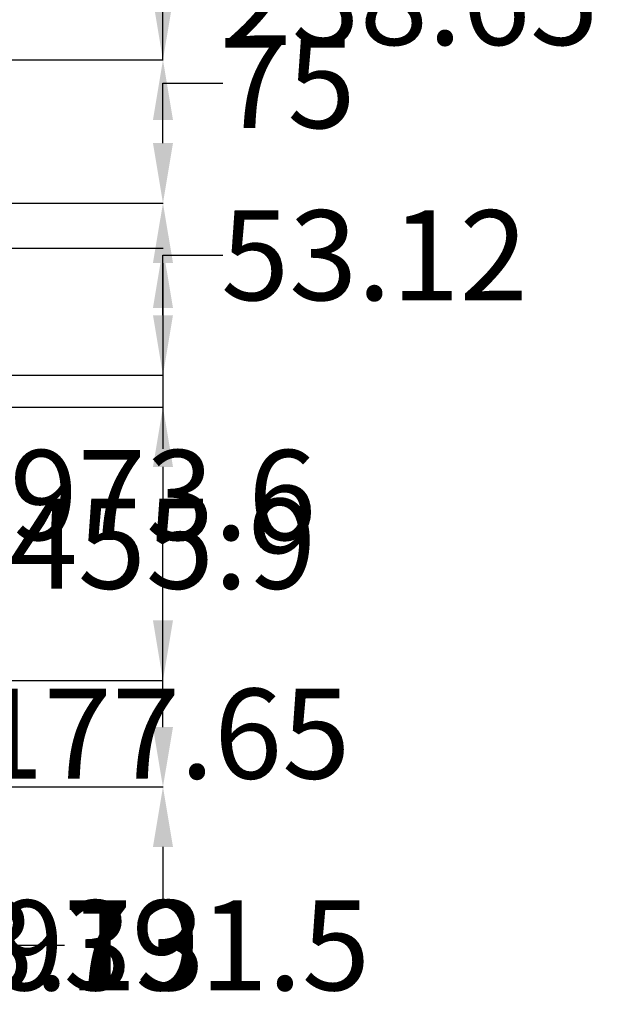
# Model space of a CAD drawing. Units: millimetres. Extents: x -504 to 6314, y 1290 to 4335.
# Tile 8 of 9: x 5350 to 6314, y 1290 to 2932. Entities that reach past the tile are written whole.
import ezdxf

# ---------------------------------------------------------------- set-up
doc = ezdxf.new("R2010")
doc.units = ezdxf.units.MM
doc.header["$MEASUREMENT"] = 0
doc.layers.add('A-ANNO-DIMS', color=2, linetype='Continuous', lineweight=18)
doc.styles.get("Standard").update_dxf_attribs({"font": 'arial.ttf'})
doc.dimstyles.get("Standard").update_dxf_attribs({"dimtxt": 150, "dimasz": 100, "dimexe": 0.18, "dimexo": 0.0625, "dimgap": 0.09, "dimtad": 0, "dimtih": 1, "dimtoh": 1, "dimdec": 0, "dimzin": 0, "dimdsep": 46, "dimtxsty": 'Standard', "dimcen": 0.09, "dimadec": 0, "dimazin": 0, "dimtfac": 1, "dimtdec": 0, "dimtofl": 0, "dimtmove": 0, "dimatfit": 3, "dimfxl": 1, "dimtolj": 1, "dimtzin": 0, "dimarcsym": 0})

# ---------------------------------------------------------------- blocks, each defined once
blk = doc.blocks.new('*D5')
at = {"layer": 'A-ANNO-DIMS', "color": 0, "lineweight": -2, "transparency": 16777216}
for p, q in [((4260.1, 2625.8), (5589, 2625.8)), ((5588.8, 2525.8), (5588.8, 2215.7)), ((5588.8, 1752.1), (5588.8, 2062.2)), ((72.9, 1652.1), (5589, 1652.1))]:
    blk.add_line(p, q, dxfattribs=at)
at = {"layer": 'A-ANNO-DIMS', "color": 0, "transparency": 16777216}
for points in [[(5572.1, 2525.8), (5605.5, 2525.8), (5588.8, 2625.8)], [(5572.1, 1752.1), (5605.5, 1752.1), (5588.8, 1652.1)]]:
    blk.add_solid(points, dxfattribs=at)
at = {"layer": 'Defpoints', "color": 0, "transparency": 16777216}
for p in [(4260, 2625.8), (5588.8, 2625.8), (72.8, 1652.1)]:
    blk.add_point(p, dxfattribs=at)
at = {"layer": 'A-ANNO-DIMS', "color": 0, "transparency": 16777216, "insert": (5588.8, 2138.9), "char_height": 150, "attachment_point": 5}
blk.add_mtext('\\A1;973.6', dxfattribs=at)
blk = doc.blocks.new('*D27')
at = {"layer": 'A-ANNO-DIMS', "color": 0, "lineweight": -2, "transparency": 16777216}
for p, q in [((5588.8, 3138.9), (5588.8, 3238.9)), ((5588.8, 3238.9), (5688.8, 3238.9)), ((5081.2, 3138.9), (5589, 3138.9)), ((5588.8, 2964.4), (5588.8, 3038.9)), ((4489, 2864.4), (5589, 2864.4))]:
    blk.add_line(p, q, dxfattribs=at)
at = {"layer": 'A-ANNO-DIMS', "color": 0, "transparency": 16777216}
for points in [[(5572.1, 3038.9), (5605.5, 3038.9), (5588.8, 3138.9)], [(5572.1, 2964.4), (5605.5, 2964.4), (5588.8, 2864.4)]]:
    blk.add_solid(points, dxfattribs=at)
at = {"layer": 'Defpoints', "color": 0, "transparency": 16777216}
for p in [(5081.2, 3138.9), (5588.8, 3138.9), (4489, 2864.4)]:
    blk.add_point(p, dxfattribs=at)
at = {"layer": 'A-ANNO-DIMS', "color": 0, "transparency": 16777216, "insert": (6001.2, 3238.9), "char_height": 150, "attachment_point": 5}
blk.add_mtext('\\A1;274.54', dxfattribs=at)
blk = doc.blocks.new('*D29')
at = {"layer": 'A-ANNO-DIMS', "color": 0, "lineweight": -2, "transparency": 16777216}
for p, q in [((5588.8, 2864.4), (5588.8, 2964.4)), ((5588.8, 2964.4), (5688.8, 2964.4)), ((4489, 2864.4), (5589, 2864.4)), ((5588.8, 2725.8), (5588.8, 2764.4)), ((4260.1, 2625.8), (5589, 2625.8))]:
    blk.add_line(p, q, dxfattribs=at)
at = {"layer": 'A-ANNO-DIMS', "color": 0, "transparency": 16777216}
for points in [[(5572.1, 2764.4), (5605.5, 2764.4), (5588.8, 2864.4)], [(5572.1, 2725.8), (5605.5, 2725.8), (5588.8, 2625.8)]]:
    blk.add_solid(points, dxfattribs=at)
at = {"layer": 'Defpoints', "color": 0, "transparency": 16777216}
for p in [(4489, 2864.4), (5588.8, 2864.4), (4260, 2625.8)]:
    blk.add_point(p, dxfattribs=at)
at = {"layer": 'A-ANNO-DIMS', "color": 0, "transparency": 16777216, "insert": (6002.1, 2964.4), "char_height": 150, "attachment_point": 5}
blk.add_mtext('\\A1;238.65', dxfattribs=at)
blk = doc.blocks.new('*D30')
at = {"layer": 'A-ANNO-DIMS', "color": 0, "lineweight": -2, "transparency": 16777216}
for p, q in [((5588.8, 2725.8), (5588.8, 2825.8)), ((5588.8, 2825.8), (5688.8, 2825.8)), ((4260.1, 2625.8), (5589, 2625.8)), ((4250.2, 2550.8), (5589, 2550.8)), ((5588.8, 2450.8), (5588.8, 2350.8))]:
    blk.add_line(p, q, dxfattribs=at)
at = {"layer": 'A-ANNO-DIMS', "color": 0, "transparency": 16777216}
for points in [[(5572.1, 2725.8), (5605.5, 2725.8), (5588.8, 2625.8)], [(5572.1, 2450.8), (5605.5, 2450.8), (5588.8, 2550.8)]]:
    blk.add_solid(points, dxfattribs=at)
at = {"layer": 'Defpoints', "color": 0, "transparency": 16777216}
for p in [(4260, 2625.8), (5588.8, 2625.8), (4250.1, 2550.8)]:
    blk.add_point(p, dxfattribs=at)
at = {"layer": 'A-ANNO-DIMS', "color": 0, "transparency": 16777216, "insert": (5796.3, 2825.8), "char_height": 150, "attachment_point": 5}
blk.add_mtext('\\A1;75', dxfattribs=at)
blk = doc.blocks.new('*D57')
at = {"layer": 'A-ANNO-DIMS', "color": 0, "lineweight": -2, "transparency": 16777216}
for p, q in [((4608.2, 2306), (4608.2, 1387.9)), ((4720.2, 2299), (4720.2, 1387.9)), ((4508.2, 1388.1), (4408.2, 1388.1)), ((4820.2, 1388.1), (4920.2, 1388.1))]:
    blk.add_line(p, q, dxfattribs=at)
at = {"layer": 'A-ANNO-DIMS', "color": 0, "transparency": 16777216}
for points in [[(4508.2, 1404.8), (4508.2, 1371.5), (4608.2, 1388.1)], [(4820.2, 1404.8), (4820.2, 1371.5), (4720.2, 1388.1)]]:
    blk.add_solid(points, dxfattribs=at)
at = {"layer": 'Defpoints', "color": 0, "transparency": 16777216}
for p in [(4608.2, 2306.1), (4720.2, 2299.1), (4720.2, 1388.1)]:
    blk.add_point(p, dxfattribs=at)
at = {"layer": 'A-ANNO-DIMS', "color": 0, "transparency": 16777216, "insert": (5224.6, 1388.1), "char_height": 150, "attachment_point": 5}
blk.add_mtext('\\A1;111.97', dxfattribs=at)
blk = doc.blocks.new('*D58')
at = {"layer": 'A-ANNO-DIMS', "color": 0, "lineweight": -2, "transparency": 16777216}
for p, q in [((4720.2, 2299), (4720.2, 1387.9)), ((4933.3, 2285.6), (4933.3, 1387.9)), ((4820.2, 1388.1), (4833.3, 1388.1)), ((4933.3, 1388.1), (5033.3, 1388.1))]:
    blk.add_line(p, q, dxfattribs=at)
at = {"layer": 'A-ANNO-DIMS', "color": 0, "transparency": 16777216}
for points in [[(4820.2, 1404.8), (4820.2, 1371.5), (4720.2, 1388.1)], [(4833.3, 1404.8), (4833.3, 1371.5), (4933.3, 1388.1)]]:
    blk.add_solid(points, dxfattribs=at)
at = {"layer": 'Defpoints', "color": 0, "transparency": 16777216}
for p in [(4720.2, 2299.1), (4933.3, 2285.7), (4933.3, 1388.1)]:
    blk.add_point(p, dxfattribs=at)
at = {"layer": 'A-ANNO-DIMS', "color": 0, "transparency": 16777216, "insert": (5346.1, 1388.1), "char_height": 150, "attachment_point": 5}
blk.add_mtext('\\A1;213.13', dxfattribs=at)
blk = doc.blocks.new('*D59')
at = {"layer": 'A-ANNO-DIMS', "color": 0, "lineweight": -2, "transparency": 16777216}
for p, q in [((4933.3, 2285.6), (4933.3, 1387.9)), ((5324.8, 2261.1), (5324.8, 1387.9)), ((5033.3, 1388.1), (5224.8, 1388.1)), ((5324.8, 1388.1), (5424.8, 1388.1))]:
    blk.add_line(p, q, dxfattribs=at)
at = {"layer": 'A-ANNO-DIMS', "color": 0, "transparency": 16777216}
for points in [[(5033.3, 1404.8), (5033.3, 1371.5), (4933.3, 1388.1)], [(5224.8, 1404.8), (5224.8, 1371.5), (5324.8, 1388.1)]]:
    blk.add_solid(points, dxfattribs=at)
at = {"layer": 'Defpoints', "color": 0, "transparency": 16777216}
for p in [(4933.3, 2285.7), (5324.8, 2261.2), (5324.8, 1388.1)]:
    blk.add_point(p, dxfattribs=at)
at = {"layer": 'A-ANNO-DIMS', "color": 0, "transparency": 16777216, "insert": (5678.5, 1388.1), "char_height": 150, "attachment_point": 5}
blk.add_mtext('\\A1;391.5', dxfattribs=at)
blk = doc.blocks.new('*D63')
at = {"layer": 'A-ANNO-DIMS', "color": 0, "lineweight": -2, "transparency": 16777216}
for p, q in [((5588.8, 1929.8), (5588.8, 2029.8)), ((3818.7, 1829.8), (5589, 1829.8)), ((3818.7, 1652.1), (5589, 1652.1)), ((5588.8, 1552.1), (5588.8, 1452.1))]:
    blk.add_line(p, q, dxfattribs=at)
at = {"layer": 'A-ANNO-DIMS', "color": 0, "transparency": 16777216}
for points in [[(5572.1, 1929.8), (5605.5, 1929.8), (5588.8, 1829.8)], [(5572.1, 1552.1), (5605.5, 1552.1), (5588.8, 1652.1)]]:
    blk.add_solid(points, dxfattribs=at)
at = {"layer": 'Defpoints', "color": 0, "transparency": 16777216}
for p in [(3818.6, 1829.8), (5588.8, 1829.8), (3818.6, 1652.1)]:
    blk.add_point(p, dxfattribs=at)
at = {"layer": 'A-ANNO-DIMS', "color": 0, "transparency": 16777216, "insert": (5588.8, 1741), "char_height": 150, "attachment_point": 5}
blk.add_mtext('\\A1;177.65', dxfattribs=at)
blk = doc.blocks.new('*D64')
at = {"layer": 'A-ANNO-DIMS', "color": 0, "lineweight": -2, "transparency": 16777216}
for p, q in [((4933.4, 2285.7), (5589, 2285.7)), ((5588.8, 2185.7), (5588.8, 2134.4)), ((5588.8, 1929.8), (5588.8, 1981.1)), ((3818.7, 1829.8), (5589, 1829.8))]:
    blk.add_line(p, q, dxfattribs=at)
at = {"layer": 'A-ANNO-DIMS', "color": 0, "transparency": 16777216}
for points in [[(5572.1, 2185.7), (5605.5, 2185.7), (5588.8, 2285.7)], [(5572.1, 1929.8), (5605.5, 1929.8), (5588.8, 1829.8)]]:
    blk.add_solid(points, dxfattribs=at)
at = {"layer": 'Defpoints', "color": 0, "transparency": 16777216}
for p in [(4933.3, 2285.7), (5588.8, 2285.7), (3818.6, 1829.8)]:
    blk.add_point(p, dxfattribs=at)
at = {"layer": 'A-ANNO-DIMS', "color": 0, "transparency": 16777216, "insert": (5588.8, 2057.7), "char_height": 150, "attachment_point": 5}
blk.add_mtext('\\A1;455.9', dxfattribs=at)
blk = doc.blocks.new('*D65')
at = {"layer": 'A-ANNO-DIMS', "color": 0, "lineweight": -2, "transparency": 16777216}
for p, q in [((5588.8, 2438.8), (5588.8, 2538.8)), ((5588.8, 2538.8), (5688.8, 2538.8)), ((5324.9, 2338.8), (5589, 2338.8)), ((4933.4, 2285.7), (5589, 2285.7)), ((5588.8, 2185.7), (5588.8, 2085.7))]:
    blk.add_line(p, q, dxfattribs=at)
at = {"layer": 'A-ANNO-DIMS', "color": 0, "transparency": 16777216}
for points in [[(5572.1, 2438.8), (5605.5, 2438.8), (5588.8, 2338.8)], [(5572.1, 2185.7), (5605.5, 2185.7), (5588.8, 2285.7)]]:
    blk.add_solid(points, dxfattribs=at)
at = {"layer": 'Defpoints', "color": 0, "transparency": 16777216}
for p in [(5324.8, 2338.8), (5588.8, 2338.8), (4933.3, 2285.7)]:
    blk.add_point(p, dxfattribs=at)
at = {"layer": 'A-ANNO-DIMS', "color": 0, "transparency": 16777216, "insert": (5941.2, 2538.8), "char_height": 150, "attachment_point": 5}
blk.add_mtext('\\A1;53.12', dxfattribs=at)

msp = doc.modelspace()

# ---------------------------------------------------------------- dimensions: what is measured, and where the dimension line sits
at = {"layer": 'A-ANNO-DIMS'}
for base, p1, p2, override, picture, middle in [((5588.7921, 3138.9408), (4488.9803, 2864.4056), (5081.1676, 3138.9408), {"dimdec": 2, "dimlfac": 1, "dimrnd": 0, "dimzin": 0, "dimdsep": 46, "dimlunit": 2}, '*D27', (6001.2116, 3238.9408)), ((5588.792, 2864.406), (4260.021, 2625.758), (4488.98, 2864.406), {"dimdec": 2, "dimlfac": 1, "dimrnd": 0, "dimzin": 0, "dimdsep": 46, "dimlunit": 2}, '*D29', (6002.081, 2964.406)), ((5588.792, 2625.758), (4250.093, 2550.758), (4260.021, 2625.758), {"dimdec": 0, "dimlfac": 1, "dimrnd": 0, "dimzin": 0, "dimdsep": 46, "dimlunit": 2}, '*D30', (5796.266, 2825.758)), ((5588.792, 2338.836), (4933.327, 2285.712), (5324.792, 2338.836), {"dimdec": 2, "dimlfac": 1, "dimrnd": 0, "dimzin": 0, "dimdsep": 46, "dimlunit": 2}, '*D65', (5941.201, 2538.836)), ((5588.792, 2625.758), (72.835, 1652.125), (4260.021, 2625.758), {"dimdec": 1, "dimlfac": 1, "dimrnd": 0, "dimzin": 0, "dimdsep": 46, "dimlunit": 2}, '*D5', (5588.792, 2138.941)), ((5588.792, 2285.712), (3818.634, 1829.779), (4933.327, 2285.712), {"dimdec": 1, "dimlfac": 1, "dimrnd": 0, "dimzin": 0, "dimdsep": 46, "dimlunit": 2}, '*D64', (5588.792, 2057.745)), ((5588.792, 1829.779), (3818.634, 1652.125), (3818.634, 1829.779), {"dimdec": 2, "dimlfac": 1, "dimrnd": 0, "dimzin": 0, "dimdsep": 46, "dimlunit": 2}, '*D63', (5588.792, 1740.952))]:
    dim = msp.add_linear_dim(base=base, p1=p1, p2=p2, angle=90, dimstyle='Standard', override=override, dxfattribs=at)
    dim.commit()
    dim.dimension.update_dxf_attribs({"geometry": picture, "text_midpoint": middle})
for base, p1, p2, override, picture, middle in [((4720.193, 1388.125), (4608.219, 2306.102), (4720.193, 2299.079), {"dimdec": 2, "dimlfac": 1, "dimrnd": 0, "dimzin": 0, "dimdsep": 46, "dimlunit": 2}, '*D57', (5224.58, 1388.125)), ((4933.327, 1388.125), (4720.193, 2299.079), (4933.327, 2285.712), {"dimdec": 2, "dimlfac": 1, "dimrnd": 0, "dimzin": 0, "dimdsep": 46, "dimlunit": 2}, '*D58', (5346.053, 1388.125)), ((5324.792, 1388.125), (4933.327, 2285.712), (5324.792, 2261.16), {"dimdec": 1, "dimlfac": 1, "dimrnd": 0, "dimzin": 0, "dimdsep": 46, "dimlunit": 2}, '*D59', (5678.48, 1388.125))]:
    dim = msp.add_linear_dim(base=base, p1=p1, p2=p2, dimstyle='Standard', override=override, dxfattribs=at)
    dim.commit()
    dim.dimension.update_dxf_attribs({"geometry": picture, "text_midpoint": middle})

doc.saveas('drawing.dxf')
